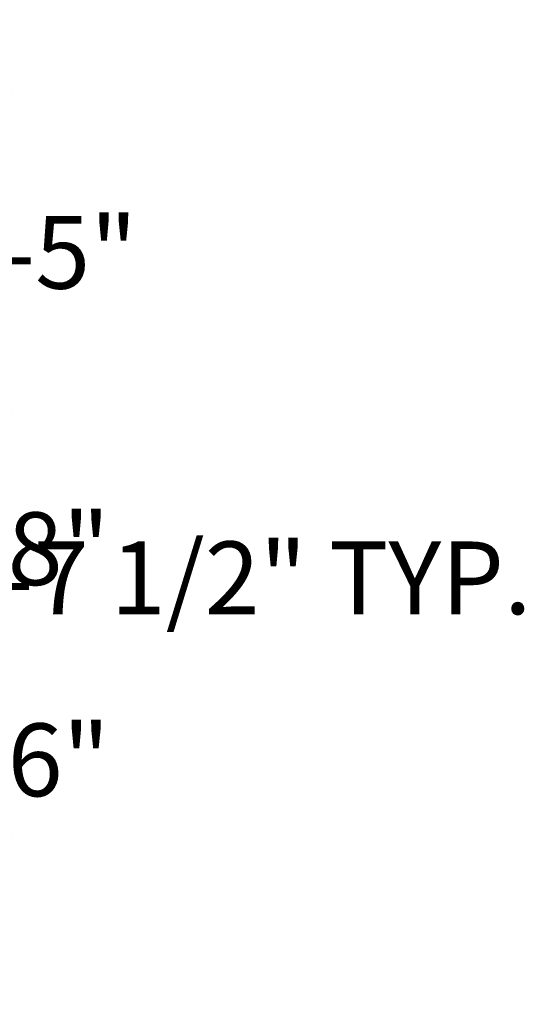
# Model space of a CAD drawing. Units: inches. Extents: x 23 to 3024, y 4 to 1405.
# Tile 7 of 7: x 2849 to 3024, y 955 to 1296. Entities that reach past the tile are written whole.
import ezdxf

# ---------------------------------------------------------------- set-up
doc = ezdxf.new("R2010")
doc.units = ezdxf.units.IN
doc.header["$MEASUREMENT"] = 0
doc.layers.add('A-ANNO-DIMS', color=2, linetype='Continuous', lineweight=18)
doc.styles.get("Standard").update_dxf_attribs({"font": 'arial.ttf'})
doc.dimstyles.get("Standard").update_dxf_attribs({"dimtxt": 25.18, "dimasz": 25.18, "dimexe": 0.18, "dimexo": 0.0625, "dimgap": 0.09, "dimtad": 0, "dimtih": 1, "dimtoh": 1, "dimdec": 0, "dimrnd": 10, "dimzin": 0, "dimdsep": 46, "dimlunit": 3, "dimtxsty": 'Standard', "dimcen": 0.09, "dimadec": 0, "dimazin": 0, "dimtfac": 1, "dimtdec": 0, "dimtofl": 0, "dimtmove": 0, "dimatfit": 3, "dimfxl": 1, "dimtolj": 1, "dimtzin": 0, "dimarcsym": 0})

# ---------------------------------------------------------------- blocks, each defined once
blk = doc.blocks.new('*D39')
at = {"layer": 'A-ANNO-DIMS', "color": 0, "lineweight": -2, "transparency": 16777216}
for p, q in [((2501.85, 1102.79), (2476.67, 1102.79)), ((2527.03, 1099.9), (2527.03, 1102.97)), ((2546.68, 1099.9), (2546.68, 1102.97)), ((2571.86, 1102.79), (2597.04, 1102.79))]:
    blk.add_line(p, q, dxfattribs=at)
at = {"layer": 'A-ANNO-DIMS', "color": 0, "transparency": 16777216}
for points in [[(2501.85, 1106.99), (2501.85, 1098.59), (2527.03, 1102.79)], [(2571.86, 1106.99), (2571.86, 1098.59), (2546.68, 1102.79)]]:
    blk.add_solid(points, dxfattribs=at)
at = {"layer": 'Defpoints', "color": 0, "transparency": 16777216}
for p in [(2546.68, 1102.79), (2527.03, 1099.84), (2546.68, 1099.84)]:
    blk.add_point(p, dxfattribs=at)
at = {"layer": 'A-ANNO-DIMS', "color": 0, "transparency": 16777216, "insert": (2816.04, 1102.79), "char_height": 25.18, "attachment_point": 5}
blk.add_mtext('\\A1;LAMP TABLE 1\'-7 1/2" TYP.', dxfattribs=at)
blk = doc.blocks.new('*D43')
at = {"layer": 'A-ANNO-DIMS', "color": 0, "lineweight": -2, "transparency": 16777216}
for p, q in [((2800.51, 1295.93), (2842.48, 1295.93)), ((2842.3, 1270.75), (2842.3, 1228.38)), ((2842.3, 1160.11), (2842.3, 1202.47)), ((2791.51, 1134.93), (2842.48, 1134.93))]:
    blk.add_line(p, q, dxfattribs=at)
at = {"layer": 'A-ANNO-DIMS', "color": 0, "transparency": 16777216}
for points in [[(2838.1, 1270.75), (2846.5, 1270.75), (2842.3, 1295.93)], [(2838.1, 1160.11), (2846.5, 1160.11), (2842.3, 1134.93)]]:
    blk.add_solid(points, dxfattribs=at)
at = {"layer": 'Defpoints', "color": 0, "transparency": 16777216}
for p in [(2800.45, 1295.93), (2791.45, 1134.93), (2842.3, 1134.93)]:
    blk.add_point(p, dxfattribs=at)
at = {"layer": 'A-ANNO-DIMS', "color": 0, "transparency": 16777216, "insert": (2842.3, 1215.43), "char_height": 25.18, "attachment_point": 5}
blk.add_mtext('\\A1;13\'-5"', dxfattribs=at)
blk = doc.blocks.new('*D45')
at = {"layer": 'A-ANNO-DIMS', "color": 0, "lineweight": -2, "transparency": 16777216}
for p, q in [((2719, 988.72), (2719, 533.9)), ((2791.45, 988.72), (2791.45, 533.9)), ((2744.18, 534.08), (2766.27, 534.08)), ((2791.45, 534.08), (2816.63, 534.08))]:
    blk.add_line(p, q, dxfattribs=at)
at = {"layer": 'A-ANNO-DIMS', "color": 0, "transparency": 16777216}
for points in [[(2744.18, 538.27), (2744.18, 529.88), (2719, 534.08)], [(2766.27, 538.27), (2766.27, 529.88), (2791.45, 534.08)]]:
    blk.add_solid(points, dxfattribs=at)
at = {"layer": 'Defpoints', "color": 0, "transparency": 16777216}
for p in [(2719, 988.78), (2791.45, 988.78), (2791.45, 534.08)]:
    blk.add_point(p, dxfattribs=at)
at = {"layer": 'A-ANNO-DIMS', "color": 0, "transparency": 16777216, "insert": (2879.59, 534.08), "char_height": 25.18, "attachment_point": 5}
blk.add_mtext('\\A1;6\'-0 1/2"', dxfattribs=at)
blk = doc.blocks.new('*D46')
at = {"layer": 'A-ANNO-DIMS', "color": 0, "lineweight": -2, "transparency": 16777216}
for p, q in [((2719.07, 1090.84), (2842.48, 1090.84)), ((2842.3, 1065.66), (2842.3, 1052.75)), ((2842.3, 1013.96), (2842.3, 1026.86)), ((2791.51, 988.78), (2842.48, 988.78))]:
    blk.add_line(p, q, dxfattribs=at)
at = {"layer": 'A-ANNO-DIMS', "color": 0, "transparency": 16777216}
for points in [[(2838.1, 1065.66), (2846.5, 1065.66), (2842.3, 1090.84)], [(2838.1, 1013.96), (2846.5, 1013.96), (2842.3, 988.78)]]:
    blk.add_solid(points, dxfattribs=at)
at = {"layer": 'Defpoints', "color": 0, "transparency": 16777216}
for p in [(2719, 1090.84), (2842.3, 1090.84), (2791.45, 988.78)]:
    blk.add_point(p, dxfattribs=at)
at = {"layer": 'A-ANNO-DIMS', "color": 0, "transparency": 16777216, "insert": (2842.3, 1039.81), "char_height": 25.18, "attachment_point": 5}
blk.add_mtext('\\A1;8\'-6"', dxfattribs=at)
blk = doc.blocks.new('*D47')
at = {"layer": 'A-ANNO-DIMS', "color": 0, "lineweight": -2, "transparency": 16777216}
for p, q in [((2842.3, 1160.11), (2842.3, 1185.29)), ((2719.07, 1134.93), (2842.48, 1134.93)), ((2719.07, 1090.84), (2842.48, 1090.84)), ((2842.3, 1065.66), (2842.3, 1040.48))]:
    blk.add_line(p, q, dxfattribs=at)
at = {"layer": 'A-ANNO-DIMS', "color": 0, "transparency": 16777216}
for points in [[(2838.1, 1160.11), (2846.5, 1160.11), (2842.3, 1134.93)], [(2838.1, 1065.66), (2846.5, 1065.66), (2842.3, 1090.84)]]:
    blk.add_solid(points, dxfattribs=at)
at = {"layer": 'Defpoints', "color": 0, "transparency": 16777216}
for p in [(2719, 1134.93), (2842.3, 1134.93), (2719, 1090.84)]:
    blk.add_point(p, dxfattribs=at)
at = {"layer": 'A-ANNO-DIMS', "color": 0, "transparency": 16777216, "insert": (2842.3, 1112.88), "char_height": 25.18, "attachment_point": 5}
blk.add_mtext('\\A1;3\'-8"', dxfattribs=at)

msp = doc.modelspace()

# ---------------------------------------------------------------- dimensions: what is measured, and where the dimension line sits
at = {"layer": 'A-ANNO-DIMS'}
for base, p1, p2, picture, middle in [((2842.3, 1134.93), (2800.45, 1295.93), (2791.45, 1134.93), '*D43', (2842.3, 1215.43)), ((2842.3, 1134.93), (2719, 1090.84), (2719, 1134.93), '*D47', (2842.3, 1112.88)), ((2842.3, 1090.84), (2791.45, 988.78), (2719, 1090.84), '*D46', (2842.3, 1039.81))]:
    dim = msp.add_linear_dim(base=base, p1=p1, p2=p2, angle=90, dimstyle='Standard', override={"dimdec": 1, "dimlfac": 1, "dimrnd": 0, "dimzin": 1, "dimdsep": 46, "dimlunit": 4, "dimfrac": 2}, dxfattribs=at)
    dim.commit()
    dim.dimension.update_dxf_attribs({"geometry": picture, "text_midpoint": middle})
dim = msp.add_linear_dim(base=(2546.6795, 1102.7891), p1=(2527.0344, 1099.8423), p2=(2546.6795, 1099.8423), text='LAMP TABLE <> TYP.', dimstyle='Standard', override={"dimdec": 1, "dimlfac": 1, "dimrnd": 0, "dimzin": 1, "dimdsep": 46, "dimlunit": 4, "dimfrac": 2}, dxfattribs=at)
dim.commit()
dim.dimension.update_dxf_attribs({"geometry": '*D39', "text_midpoint": (2816.0374, 1102.7891)})
dim = msp.add_linear_dim(base=(2791.449, 534.0772), p1=(2719.0035, 988.7789), p2=(2791.449, 988.7789), dimstyle='Standard', override={"dimdec": 1, "dimlfac": 1, "dimrnd": 0, "dimzin": 1, "dimdsep": 46, "dimlunit": 4, "dimfrac": 2}, dxfattribs=at)
dim.commit()
dim.dimension.update_dxf_attribs({"geometry": '*D45', "text_midpoint": (2879.5917, 534.0772)})

doc.saveas('drawing.dxf')
